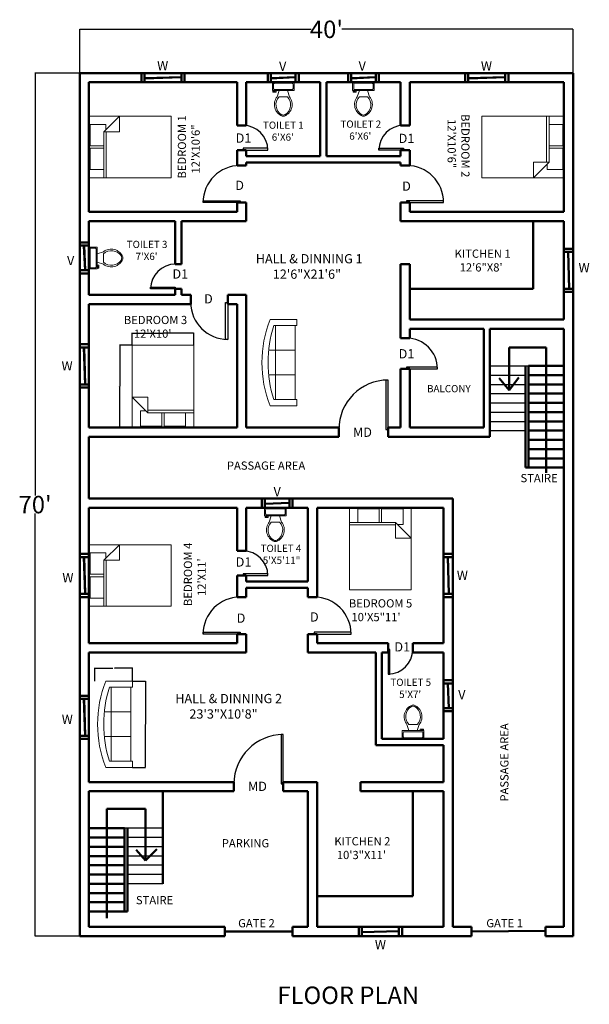
# Model space of a CAD drawing. Units: inches. Extents: x 9239 to 26065, y 6728 to 14611.
# Tile 5 of 12: x 11268 to 11822, y 6974 to 7933. Entities that reach past the tile are written whole.
import ezdxf

# ---------------------------------------------------------------- set-up
doc = ezdxf.new("R2010")
doc.units = ezdxf.units.IN
doc.header["$MEASUREMENT"] = 0
for name, color, linetype, lineweight in [('A-ANNO-DIMS', 2, 'Continuous', 18), ('A-ANNO-TEXT', 7, 'Continuous', 18), ('A-AREA-IDEN', 7, 'Continuous', 18), ('A-DOOR', 4, 'Continuous', 25), ('A-FLOR-FIXT', 8, 'Continuous', 18), ('A-FLOR-STRS', 3, 'Continuous', 25), ('A-FURN', 8, 'Continuous', 18), ('A-GLAZ', 4, 'Continuous', 25), ('A-WALL', 7, 'Continuous', 50)]:
    doc.layers.add(name, color=color, linetype=linetype, lineweight=lineweight)
doc.styles.get("Standard").update_dxf_attribs({"font": 'arial.ttf'})
doc.dimstyles.get("Standard").update_dxf_attribs({"dimtxt": 0.18, "dimasz": 0.18, "dimexe": 0.18, "dimexo": 0.0625, "dimgap": 0.09, "dimtad": 0, "dimtih": 1, "dimtoh": 1, "dimdec": 0, "dimzin": 0, "dimdsep": 46, "dimlunit": 3, "dimtxsty": 'Standard', "dimcen": 0.09, "dimadec": 0, "dimazin": 0, "dimtfac": 1, "dimtdec": 0, "dimtofl": 0, "dimtmove": 0, "dimatfit": 3, "dimfxl": 1, "dimtolj": 1, "dimtzin": 0, "dimarcsym": 0})

# ---------------------------------------------------------------- blocks, each defined once
blk = doc.blocks.new('Bed - Queen')
for p, q in [((0, -80.00003), (0, 0)), ((0, 0), (59.99999, 0)), ((59.99999, 0), (59.99999, -80.00003)), ((7.99999, -1.2), (28.79998, -1.2)), ((7.99999, -14.4), (7.99999, -1.2)), ((28.79998, -1.2), (28.79998, -14.4)), ((31.19999, -1.2), (51.99999, -1.2)), ((31.19999, -14.4), (31.19999, -1.2)), ((51.99999, -1.2), (51.99999, -16.4)), ((0, -14.4), (44.8, -14.4)), ((44.8, -16.8), (0, -16.8)), ((59.99999, -29.6), (44.8, -14.4)), ((44.8, -14.4), (44.8, -29.6)), ((51.99999, -16.4), (46.79936, -16.4)), ((44.8, -29.6), (59.99999, -29.6)), ((59.99999, -80.00003), (0, -80.00003))]:
    blk.add_line(p, q)
blk = doc.blocks.new('Sofa - Roundback 7 ft.')
for p, q in [((-12.00002, -32.4421), (-12.00003, -6.5971)), ((11.99997, -32.4421), (11.99998, -6.5971)), ((-36.000027, -34), (-36.000027, -11.4696)), ((-35.999844, -13.3819), (35.9998, -13.3819)), ((35.99998, -34), (35.99998, -11.4696)), ((-36.000027, -32.4421), (35.99998, -32.4421))]:
    blk.add_line(p, q)
for points in [[(-36.000027, -34), (-42.000027, -34), (-42.000027, -8)], [(41.99998, -8), (41.99998, -34), (35.99998, -34)]]:
    blk.add_lwpolyline(points)
for centre, radius, start, end in [((0, -114.25), 114.25, 68.43141, 111.5686), ((-0.00001, -127.1968), 121.1968, 72.72033, 107.2797)]:
    blk.add_arc(centre, radius, start, end)
blk = doc.blocks.new('Toilet - top')
for p, q in [((-10, -8.5), (-8, -8.5)), ((-10, -9.5), (-10, -8.5)), ((-7, -9.5), (-10, -9.5)), ((-8, -8.5), (-8, -8)), ((-7, -8), (-7, -9.5)), ((-4, -8), (-6, -14)), ((4, -8), (6, -14)), ((9.5, -6), (9.5, -2)), ((4, -14), (-4, -14))]:
    blk.add_line(p, q)
blk.add_lwpolyline([(10.5, -8), (10.5, 0), (-10.5, 0), (-10.5, -8)], close=True)
for points in [[(-9.5, -2), (-9.5, -6)], [(8.5, -1), (-8.5, -1)], [(-8.5, -7), (8.5, -7)]]:
    blk.add_lwpolyline(points)
for centre, radius, start, end in [((-8.62, -1.88), 0.884, 81.8699, 188.1301), ((-8.62, -6.12), 0.884, 171.8699, 278.1301), ((8.62, -1.88), 0.884, 351.8699, 98.1301), ((8.62, -6.12), 0.884, 261.8699, 8.1301), ((3.52, -21.58), 12.17, 141.46911, 247.97143), ((4.2, -21.82), 11.33, 136.36773, 238.94682), ((-3.52, -21.58), 12.17, 292.02843, 38.53071), ((-4.2, -21.82), 11.33, 301.05301, 43.63209), ((0, -27.88), 4, 245.73182, 294.26817), ((0, -29), 4, 254.86053, 285.13947)]:
    blk.add_arc(centre, radius, start, end)
blk = doc.blocks.new('*U16')
for p, q in [((0, 0), (0, -6)), ((-40, 0), (-40, -6))]:
    blk.add_line(p, q)
blk.add_lwpolyline([(0, 0), (0, 40), (-1.75, 40), (-1.75, 0)], close=True)
blk.add_arc((0, 0), 40, 90, 180)
blk = doc.blocks.new('*U11')
for p, q in [((0, 0), (0, -6)), ((-36, 0), (-36, -6))]:
    blk.add_line(p, q)
blk.add_lwpolyline([(0, 0), (0, 36), (-1.75, 36), (-1.75, 0)], close=True)
blk.add_arc((0, 0), 36, 90, 180)
blk = doc.blocks.new('*U25')
for p, q in [((-24, 0), (-24, -6)), ((0, 0), (0, -6))]:
    blk.add_line(p, q)
blk.add_lwpolyline([(0, 0), (0, 24), (-1.75, 24), (-1.75, 0)], close=True)
blk.add_arc((0, 0), 24, 90, 180)
blk = doc.blocks.new('*U24')
for p, q in [((0, 0), (0, 6)), ((24, 0), (24, 6))]:
    blk.add_line(p, q)
blk.add_lwpolyline([(0, 0), (0, -24), (1.75, -24), (1.75, 0)], close=True)
blk.add_arc((0, 0), 24, 270, 0)
blk = doc.blocks.new('*U14')
for p, q in [((-36, 0), (-36, 6)), ((0, 0), (0, 6))]:
    blk.add_line(p, q)
blk.add_lwpolyline([(0, 0), (0, -36), (-1.75, -36), (-1.75, 0)], close=True)
blk.add_arc((0, 0), 36, 180, 270)
blk = doc.blocks.new('*U29')
for p, q in [((-24, 0), (-24, 6)), ((0, 0), (0, 6))]:
    blk.add_line(p, q)
blk.add_lwpolyline([(0, 0), (0, -24), (-1.75, -24), (-1.75, 0)], close=True)
blk.add_arc((0, 0), 24, 180, 270)
blk = doc.blocks.new('*U26')
for p, q in [((-24, 0), (-24, -6)), ((0, 0), (0, -6))]:
    blk.add_line(p, q)
blk.add_lwpolyline([(0, 0), (0, 24), (-1.75, 24), (-1.75, 0)], close=True)
blk.add_arc((0, 0), 24, 90, 180)
blk = doc.blocks.new('*U30')
for p, q in [((0, 0), (0, -6)), ((-36, 0), (-36, -6))]:
    blk.add_line(p, q)
blk.add_lwpolyline([(0, 0), (0, 36), (-1.75, 36), (-1.75, 0)], close=True)
blk.add_arc((0, 0), 36, 90, 180)
blk = doc.blocks.new('*U28')
for p, q in [((0, 0), (0, -6)), ((-30, 0), (-30, -6))]:
    blk.add_line(p, q)
blk.add_lwpolyline([(0, 0), (0, 30), (-1.75, 30), (-1.75, 0)], close=True)
blk.add_arc((0, 0), 30, 90, 180)
blk = doc.blocks.new('*U27')
for p, q in [((-30, 0), (-30, 6)), ((0, 0), (0, 6))]:
    blk.add_line(p, q)
blk.add_lwpolyline([(0, 0), (0, -30), (-1.75, -30), (-1.75, 0)], close=True)
blk.add_arc((0, 0), 30, 180, 270)
blk = doc.blocks.new('*D31')
at = {"layer": 'A-ANNO-DIMS', "color": 0, "lineweight": -2, "transparency": 16777216}
for p, q in [((11326.22, 7880.73), (11326.22, 7923.38)), ((11326.4, 7923.2), (11551.37, 7923.2)), ((11806.04, 7923.2), (11581.08, 7923.2)), ((11806.22, 7880.73), (11806.22, 7923.38))]:
    blk.add_line(p, q, dxfattribs=at)
at = {"layer": 'A-ANNO-DIMS', "color": 0, "transparency": 16777216}
for points in [[(11326.4, 7923.23), (11326.4, 7923.17), (11326.22, 7923.2)], [(11806.04, 7923.23), (11806.04, 7923.17), (11806.22, 7923.2)]]:
    blk.add_solid(points, dxfattribs=at)
at = {"layer": 'Defpoints', "color": 0, "transparency": 16777216}
for p in [(11806.22, 7923.2), (11326.22, 7880.66), (11806.22, 7880.66)]:
    blk.add_point(p, dxfattribs=at)
at = {"layer": 'A-ANNO-DIMS', "color": 0, "transparency": 16777216, "insert": (11566.22, 7923.2), "char_height": 0.18, "attachment_point": 5}
blk.add_mtext("\\A1;{\\H94.44444x;40'}", dxfattribs=at)
blk = doc.blocks.new('*D32')
at = {"layer": 'A-ANNO-DIMS', "color": 0, "lineweight": -2, "transparency": 16777216}
for p, q in [((11326.16, 7880.66), (11282.62, 7880.66)), ((11282.8, 7880.48), (11282.8, 7469.43)), ((11282.8, 7040.84), (11282.8, 7451.89)), ((11326.16, 7040.66), (11282.62, 7040.66))]:
    blk.add_line(p, q, dxfattribs=at)
at = {"layer": 'A-ANNO-DIMS', "color": 0, "transparency": 16777216}
for points in [[(11282.77, 7880.48), (11282.83, 7880.48), (11282.8, 7880.66)], [(11282.77, 7040.84), (11282.83, 7040.84), (11282.8, 7040.66)]]:
    blk.add_solid(points, dxfattribs=at)
at = {"layer": 'Defpoints', "color": 0, "transparency": 16777216}
for p in [(11326.22, 7880.66), (11282.8, 7040.66), (11326.22, 7040.66)]:
    blk.add_point(p, dxfattribs=at)
at = {"layer": 'A-ANNO-DIMS', "color": 0, "transparency": 16777216, "insert": (11282.8, 7460.66), "char_height": 0.18, "width": 0.304, "attachment_point": 5}
blk.add_mtext("\\A1;{\\H94.44444x;70'}", dxfattribs=at)
blk = doc.blocks.new('WIN-36')
for p, q in [((0, 1), (36, 1)), ((0, 0.5), (36, 0.5)), ((0, 0), (36, 0))]:
    blk.add_line(p, q)
blk = doc.blocks.new('WIN-24')
for p, q in [((0, 1), (24, 1)), ((0, 0.5), (24, 0.5)), ((0, 0), (24, 0))]:
    blk.add_line(p, q)
blk = doc.blocks.new('*D46')
at = {"layer": 'A-ANNO-DIMS', "color": 0, "lineweight": -2, "transparency": 16777216}
for p, q in [((11377.16, 7615.66), (11365.04, 7615.66)), ((11365.22, 7615.48), (11365.22, 7575.85)), ((11365.22, 7535.84), (11365.22, 7575.48)), ((11377.16, 7535.66), (11365.04, 7535.66))]:
    blk.add_line(p, q, dxfattribs=at)
at = {"layer": 'A-ANNO-DIMS', "color": 0, "transparency": 16777216}
for points in [[(11365.19, 7615.48), (11365.25, 7615.48), (11365.22, 7615.66)], [(11365.19, 7535.84), (11365.25, 7535.84), (11365.22, 7535.66)]]:
    blk.add_solid(points, dxfattribs=at)
at = {"layer": 'Defpoints', "color": 0, "transparency": 16777216}
for p in [(11377.22, 7615.66), (11365.22, 7535.66), (11377.22, 7535.66)]:
    blk.add_point(p, dxfattribs=at)
at = {"layer": 'A-ANNO-DIMS', "color": 0, "transparency": 16777216, "insert": (11365.22, 7575.66), "char_height": 0.18, "attachment_point": 5}
blk.add_mtext('\\A1;QUEEN BED 6\'-8" TYP.', dxfattribs=at)
blk = doc.blocks.new('*D47')
at = {"layer": 'A-ANNO-DIMS', "color": 0, "lineweight": -2, "transparency": 16777216}
for p, q in [((11377.22, 7615.73), (11377.22, 7627.84)), ((11377.4, 7627.66), (11406.59, 7627.66)), ((11437.04, 7627.66), (11407.86, 7627.66)), ((11437.22, 7615.73), (11437.22, 7627.84))]:
    blk.add_line(p, q, dxfattribs=at)
at = {"layer": 'A-ANNO-DIMS', "color": 0, "transparency": 16777216}
for points in [[(11377.4, 7627.69), (11377.4, 7627.63), (11377.22, 7627.66)], [(11437.04, 7627.69), (11437.04, 7627.63), (11437.22, 7627.66)]]:
    blk.add_solid(points, dxfattribs=at)
at = {"layer": 'Defpoints', "color": 0, "transparency": 16777216}
for p in [(11377.22, 7627.66), (11377.22, 7615.66), (11437.22, 7615.66)]:
    blk.add_point(p, dxfattribs=at)
at = {"layer": 'A-ANNO-DIMS', "color": 0, "transparency": 16777216, "insert": (11407.22, 7627.66), "char_height": 0.18, "attachment_point": 5}
blk.add_mtext('\\A1;5\'-0" TYP.', dxfattribs=at)
blk = doc.blocks.new('*D54')
at = {"layer": 'A-ANNO-DIMS', "color": 0, "lineweight": -2, "transparency": 16777216}
for p, q in [((11377.64, 7288.88), (11390.36, 7288.88)), ((11390.18, 7288.7), (11390.18, 7247.06)), ((11390.18, 7205.06), (11390.18, 7246.7)), ((11377.64, 7204.88), (11390.36, 7204.88))]:
    blk.add_line(p, q, dxfattribs=at)
at = {"layer": 'A-ANNO-DIMS', "color": 0, "transparency": 16777216}
for points in [[(11390.15, 7288.7), (11390.21, 7288.7), (11390.18, 7288.88)], [(11390.15, 7205.06), (11390.21, 7205.06), (11390.18, 7204.88)]]:
    blk.add_solid(points, dxfattribs=at)
at = {"layer": 'Defpoints', "color": 0, "transparency": 16777216}
for p in [(11377.58, 7288.88), (11390.18, 7288.88), (11377.58, 7204.88)]:
    blk.add_point(p, dxfattribs=at)
at = {"layer": 'A-ANNO-DIMS', "color": 0, "transparency": 16777216, "insert": (11390.18, 7246.88), "char_height": 0.18, "attachment_point": 5}
blk.add_mtext('\\A1;SOFA 7\'-0" TYP.', dxfattribs=at)
blk = doc.blocks.new('*D55')
at = {"layer": 'A-ANNO-DIMS', "color": 0, "lineweight": -2, "transparency": 16777216}
for p, q in [((11340.91, 7288.94), (11340.91, 7301.66)), ((11341.09, 7301.48), (11358.4, 7301.48)), ((11377.4, 7301.48), (11360.09, 7301.48)), ((11377.58, 7288.94), (11377.58, 7301.66))]:
    blk.add_line(p, q, dxfattribs=at)
at = {"layer": 'A-ANNO-DIMS', "color": 0, "transparency": 16777216}
for points in [[(11341.09, 7301.51), (11341.09, 7301.45), (11340.91, 7301.48)], [(11377.4, 7301.51), (11377.4, 7301.45), (11377.58, 7301.48)]]:
    blk.add_solid(points, dxfattribs=at)
at = {"layer": 'Defpoints', "color": 0, "transparency": 16777216}
for p in [(11340.91, 7301.48), (11340.91, 7288.88), (11377.58, 7288.88)]:
    blk.add_point(p, dxfattribs=at)
at = {"layer": 'A-ANNO-DIMS', "color": 0, "transparency": 16777216, "insert": (11359.25, 7301.48), "char_height": 0.18, "attachment_point": 5}
blk.add_mtext('\\A1;3\'-0 1/2" TYP.', dxfattribs=at)

msp = doc.modelspace()

# ---------------------------------------------------------------- linework, layer by layer
at = {"layer": 'A-FLOR-STRS'}
for p, q in [((11725.22, 7595.66), (11762.72, 7595.66)), ((11725.22, 7586.66), (11759.72, 7586.66)), ((11725.22, 7577.66), (11759.72, 7577.66)), ((11725.22, 7568.66), (11759.72, 7568.66)), ((11725.22, 7559.66), (11759.72, 7559.66)), ((11725.22, 7550.66), (11759.72, 7550.66)), ((11725.22, 7541.66), (11759.72, 7541.66)), ((11725.22, 7532.66), (11759.72, 7532.66)), ((11407.22, 7145.66), (11369.72, 7145.66)), ((11407.22, 7136.66), (11372.72, 7136.66)), ((11407.22, 7127.66), (11372.72, 7127.66)), ((11407.22, 7118.66), (11372.72, 7118.66)), ((11407.22, 7109.66), (11372.72, 7109.66)), ((11407.22, 7100.66), (11372.72, 7100.66)), ((11407.22, 7091.66), (11372.72, 7091.66))]:
    msp.add_line(p, q, dxfattribs=at)
at = {"layer": 'A-WALL'}
for p, q in [((11326.22, 7880.66), (11806.22, 7880.66)), ((11326.22, 7040.66), (11326.22, 7880.66)), ((11386.22, 7871.66), (11386.22, 7880.66)), ((11389.22, 7871.66), (11389.22, 7880.66)), ((11425.22, 7871.66), (11425.22, 7880.66)), ((11428.22, 7871.66), (11428.22, 7880.66)), ((11509.22, 7871.66), (11509.22, 7880.66)), ((11512.22, 7871.66), (11512.22, 7880.66)), ((11536.22, 7871.66), (11536.22, 7880.66)), ((11539.22, 7871.66), (11539.22, 7880.66)), ((11587.22, 7871.66), (11587.22, 7880.66)), ((11590.22, 7871.66), (11590.22, 7880.66)), ((11614.22, 7871.66), (11614.22, 7880.66)), ((11617.22, 7871.66), (11617.22, 7880.66)), ((11701.22, 7871.66), (11701.22, 7880.66)), ((11704.22, 7871.66), (11704.22, 7880.66)), ((11740.22, 7871.66), (11740.22, 7880.66)), ((11743.22, 7871.66), (11743.22, 7880.66)), ((11806.22, 7880.66), (11806.22, 7040.66)), ((11335.22, 7871.66), (11479.22, 7871.66)), ((11335.22, 7745.66), (11335.22, 7871.66)), ((11479.22, 7829.66), (11479.22, 7871.66)), ((11488.22, 7829.66), (11488.22, 7871.66)), ((11488.22, 7871.66), (11560.22, 7871.66)), ((11560.22, 7799.66), (11560.22, 7871.66)), ((11566.22, 7799.66), (11566.22, 7871.66)), ((11566.22, 7871.66), (11638.22, 7871.66)), ((11638.22, 7829.66), (11638.22, 7871.66)), ((11647.22, 7829.66), (11647.22, 7871.66)), ((11647.22, 7871.66), (11797.22, 7871.66)), ((11797.22, 7871.66), (11797.22, 7745.66)), ((11479.22, 7829.66), (11488.22, 7829.66)), ((11638.22, 7829.66), (11647.22, 7829.66)), ((11479.22, 7790.66), (11479.22, 7805.66)), ((11479.22, 7805.66), (11488.22, 7805.66)), ((11488.22, 7799.66), (11488.22, 7805.66)), ((11638.22, 7805.66), (11647.22, 7805.66)), ((11638.22, 7799.66), (11638.22, 7805.66)), ((11647.22, 7790.66), (11647.22, 7805.66)), ((11479.22, 7790.66), (11488.22, 7790.66)), ((11488.22, 7799.66), (11560.22, 7799.66)), ((11488.22, 7793.66), (11638.22, 7793.66)), ((11488.22, 7790.66), (11488.22, 7793.66)), ((11566.22, 7799.66), (11638.22, 7799.66)), ((11638.22, 7790.66), (11638.22, 7793.66)), ((11638.22, 7790.66), (11647.22, 7790.66)), ((11479.22, 7745.66), (11479.22, 7754.66)), ((11479.22, 7754.66), (11488.22, 7754.66)), ((11488.22, 7736.66), (11488.22, 7754.66)), ((11638.22, 7736.66), (11638.22, 7754.66)), ((11638.22, 7754.66), (11647.22, 7754.66)), ((11647.22, 7745.66), (11647.22, 7754.66)), ((11335.22, 7745.66), (11479.22, 7745.66)), ((11647.22, 7745.66), (11797.22, 7745.66)), ((11335.22, 7736.66), (11419.22, 7736.66)), ((11335.22, 7664.66), (11335.22, 7736.66)), ((11419.22, 7694.66), (11419.22, 7736.66)), ((11425.22, 7694.66), (11425.22, 7736.66)), ((11425.22, 7736.66), (11488.22, 7736.66)), ((11638.22, 7736.66), (11797.22, 7736.66)), ((11767.22, 7736.66), (11767.22, 7670.66)), ((11797.22, 7736.66), (11797.22, 7640.66)), ((11335.22, 7715.66), (11326.22, 7715.66)), ((11335.22, 7712.66), (11326.22, 7712.66)), ((11797.22, 7709.66), (11806.22, 7709.66)), ((11797.22, 7706.66), (11806.22, 7706.66)), ((11335.22, 7688.66), (11326.22, 7688.66)), ((11335.22, 7685.66), (11326.22, 7685.66)), ((11419.22, 7694.66), (11425.22, 7694.66)), ((11638.22, 7694.66), (11647.22, 7694.66)), ((11638.22, 7622.66), (11638.22, 7694.66)), ((11647.22, 7640.66), (11647.22, 7694.66)), ((11419.22, 7664.66), (11419.22, 7670.66)), ((11419.22, 7670.66), (11425.22, 7670.66)), ((11425.22, 7664.66), (11425.22, 7670.66)), ((11647.22, 7670.66), (11767.22, 7670.66)), ((11797.22, 7670.66), (11806.22, 7670.66)), ((11797.22, 7667.66), (11806.22, 7667.66)), ((11335.22, 7664.66), (11419.22, 7664.66)), ((11425.22, 7664.66), (11434.22, 7664.66)), ((11434.22, 7655.66), (11434.22, 7664.66)), ((11470.22, 7655.66), (11470.22, 7664.66)), ((11470.22, 7664.66), (11488.22, 7664.66)), ((11488.22, 7535.66), (11488.22, 7664.66)), ((11335.22, 7655.66), (11434.22, 7655.66)), ((11335.22, 7535.66), (11335.22, 7655.66)), ((11470.22, 7655.66), (11479.22, 7655.66)), ((11479.22, 7535.66), (11479.22, 7655.66)), ((11647.22, 7640.66), (11797.22, 7640.66)), ((11647.22, 7631.66), (11719.22, 7631.66)), ((11647.22, 7622.66), (11647.22, 7631.66)), ((11719.22, 7631.66), (11719.22, 7535.66)), ((11725.22, 7631.66), (11725.22, 7526.66)), ((11725.22, 7631.66), (11797.22, 7631.66)), ((11797.22, 7631.66), (11797.22, 7049.66)), ((11638.22, 7622.66), (11647.22, 7622.66)), ((11335.22, 7616.66), (11326.22, 7616.66)), ((11335.22, 7613.66), (11326.22, 7613.66)), ((11779.97, 7613.53), (11743.89, 7613.53)), ((11743.89, 7613.53), (11743.89, 7571.97)), ((11779.97, 7491.45), (11779.97, 7613.53)), ((11638.22, 7571.66), (11638.22, 7592.66)), ((11638.22, 7592.66), (11647.22, 7592.66)), ((11647.22, 7571.66), (11647.22, 7592.66)), ((11759.72, 7595.66), (11759.72, 7496.66)), ((11762.72, 7595.66), (11762.72, 7496.66)), ((11762.72, 7595.66), (11797.22, 7595.66)), ((11743.89, 7571.97), (11734.18, 7583.85)), ((11743.89, 7571.97), (11753.43, 7584.48)), ((11762.72, 7586.66), (11797.22, 7586.66)), ((11335.22, 7577.66), (11326.22, 7577.66)), ((11335.22, 7574.66), (11326.22, 7574.66)), ((11638.22, 7535.66), (11638.22, 7571.66)), ((11647.22, 7535.66), (11647.22, 7571.66)), ((11762.72, 7577.66), (11797.22, 7577.66)), ((11762.72, 7568.66), (11797.22, 7568.66)), ((11762.72, 7559.66), (11797.22, 7559.66)), ((11762.72, 7550.66), (11797.22, 7550.66)), ((11762.72, 7541.66), (11797.22, 7541.66)), ((11335.22, 7535.66), (11479.22, 7535.66)), ((11488.22, 7535.66), (11578.22, 7535.66)), ((11578.22, 7526.66), (11578.22, 7535.66)), ((11626.22, 7526.66), (11626.22, 7535.66)), ((11626.22, 7535.66), (11638.22, 7535.66)), ((11647.22, 7535.66), (11719.22, 7535.66)), ((11762.72, 7532.66), (11797.22, 7532.66)), ((11335.22, 7526.66), (11578.22, 7526.66)), ((11335.22, 7466.66), (11335.22, 7526.66)), ((11626.22, 7526.66), (11725.22, 7526.66)), ((11762.72, 7523.66), (11797.22, 7523.66)), ((11762.72, 7514.66), (11797.22, 7514.66)), ((11762.72, 7505.66), (11797.22, 7505.66)), ((11759.72, 7496.66), (11797.22, 7496.66)), ((11335.22, 7466.66), (11689.22, 7466.66)), ((11503.22, 7457.66), (11503.22, 7466.66)), ((11506.22, 7457.66), (11506.22, 7466.66)), ((11530.22, 7457.66), (11530.22, 7466.66)), ((11533.22, 7457.66), (11533.22, 7466.66)), ((11689.22, 7466.66), (11689.22, 7049.66)), ((11335.22, 7457.66), (11479.22, 7457.66)), ((11335.22, 7325.66), (11335.22, 7457.66)), ((11476.22, 7457.66), (11479.22, 7457.66)), ((11479.22, 7415.66), (11479.22, 7457.66)), ((11488.22, 7415.66), (11488.22, 7457.66)), ((11488.22, 7457.66), (11548.22, 7457.66)), ((11548.22, 7385.66), (11548.22, 7457.66)), ((11557.22, 7370.66), (11557.22, 7457.66)), ((11557.22, 7457.66), (11680.22, 7457.66)), ((11680.22, 7457.66), (11680.22, 7325.66)), ((11335.22, 7412.66), (11326.22, 7412.66)), ((11335.22, 7409.66), (11326.22, 7409.66)), ((11479.22, 7415.66), (11488.22, 7415.66)), ((11680.22, 7412.66), (11689.22, 7412.66)), ((11680.22, 7409.66), (11689.22, 7409.66)), ((11479.22, 7370.66), (11479.22, 7391.66)), ((11479.22, 7391.66), (11488.22, 7391.66)), ((11488.22, 7385.66), (11488.22, 7391.66)), ((11488.22, 7385.66), (11548.22, 7385.66)), ((11488.22, 7379.66), (11548.22, 7379.66)), ((11488.22, 7370.66), (11488.22, 7379.66)), ((11548.22, 7370.66), (11548.22, 7379.66)), ((11335.22, 7373.66), (11326.22, 7373.66)), ((11335.22, 7370.66), (11326.22, 7370.66)), ((11479.22, 7370.66), (11488.22, 7370.66)), ((11548.22, 7370.66), (11557.22, 7370.66)), ((11680.22, 7373.66), (11689.22, 7373.66)), ((11680.22, 7370.66), (11689.22, 7370.66)), ((11479.22, 7334.66), (11488.22, 7334.66)), ((11479.22, 7325.66), (11479.22, 7334.66)), ((11488.22, 7316.66), (11488.22, 7334.66)), ((11548.22, 7316.66), (11548.22, 7334.66)), ((11548.22, 7334.66), (11557.22, 7334.66)), ((11557.22, 7325.66), (11557.22, 7334.66)), ((11335.22, 7325.66), (11479.22, 7325.66)), ((11557.22, 7325.66), (11626.22, 7325.66)), ((11626.22, 7325.66), (11626.22, 7316.66)), ((11650.22, 7325.66), (11650.22, 7316.66)), ((11650.22, 7325.66), (11680.22, 7325.66)), ((11335.22, 7316.66), (11488.22, 7316.66)), ((11335.22, 7190.66), (11335.22, 7316.66)), ((11548.22, 7316.66), (11614.22, 7316.66)), ((11614.22, 7316.66), (11614.22, 7226.66)), ((11620.22, 7316.66), (11620.22, 7232.66)), ((11620.22, 7316.66), (11626.22, 7316.66)), ((11650.22, 7316.66), (11680.22, 7316.66)), ((11680.22, 7316.66), (11680.22, 7232.66)), ((11680.22, 7289.66), (11689.22, 7289.66)), ((11680.22, 7286.66), (11689.22, 7286.66)), ((11335.22, 7274.66), (11326.22, 7274.66)), ((11335.22, 7271.66), (11326.22, 7271.66)), ((11680.22, 7262.66), (11689.22, 7262.66)), ((11680.22, 7259.66), (11689.22, 7259.66)), ((11335.22, 7235.66), (11326.22, 7235.66)), ((11335.22, 7232.66), (11326.22, 7232.66)), ((11614.22, 7226.66), (11680.22, 7226.66)), ((11620.22, 7232.66), (11680.22, 7232.66)), ((11680.22, 7226.66), (11680.22, 7190.66)), ((11476.22, 7190.66), (11335.22, 7190.66)), ((11476.22, 7181.66), (11476.22, 7190.66)), ((11557.22, 7190.66), (11524.22, 7190.66)), ((11557.22, 7190.66), (11524.22, 7190.66)), ((11524.22, 7181.66), (11524.22, 7190.66)), ((11557.22, 7049.66), (11557.22, 7190.66)), ((11680.22, 7190.66), (11599.22, 7190.66)), ((11599.22, 7181.66), (11599.22, 7190.66)), ((11335.22, 7049.66), (11335.22, 7181.66)), ((11476.22, 7181.66), (11335.22, 7181.66)), ((11407.22, 7091.66), (11407.22, 7181.66)), ((11548.22, 7181.66), (11524.22, 7181.66)), ((11548.22, 7049.66), (11548.22, 7181.66)), ((11680.22, 7181.66), (11599.22, 7181.66)), ((11650.22, 7181.66), (11650.22, 7079.66)), ((11680.22, 7181.66), (11680.22, 7049.66)), ((11352.47, 7058.27), (11352.47, 7164.58)), ((11352.47, 7164.58), (11390.09, 7164.58)), ((11390.09, 7164.58), (11390.09, 7114.39)), ((11369.72, 7145.66), (11335.22, 7145.66)), ((11369.72, 7064.66), (11369.72, 7145.66)), ((11372.72, 7064.66), (11372.72, 7145.66)), ((11369.72, 7136.66), (11335.22, 7136.66)), ((11369.72, 7127.66), (11335.22, 7127.66)), ((11390.09, 7114.39), (11381, 7124.81)), ((11390.09, 7114.39), (11401.25, 7125.18)), ((11369.72, 7118.66), (11335.22, 7118.66)), ((11369.72, 7109.66), (11335.22, 7109.66)), ((11369.72, 7100.66), (11335.22, 7100.66)), ((11369.72, 7091.66), (11335.22, 7091.66)), ((11369.72, 7082.66), (11335.22, 7082.66)), ((11369.72, 7073.66), (11335.22, 7073.66)), ((11650.22, 7079.66), (11557.22, 7079.66)), ((11372.72, 7064.66), (11335.22, 7064.66)), ((11467.22, 7049.66), (11335.22, 7049.66)), ((11467.22, 7049.66), (11467.22, 7040.66)), ((11467.22, 7045.16), (11533.22, 7045.16)), ((11548.22, 7049.66), (11533.22, 7049.66)), ((11533.22, 7040.66), (11533.22, 7049.66)), ((11680.22, 7049.66), (11557.22, 7049.66)), ((11597.72, 7049.66), (11597.72, 7040.66)), ((11600.72, 7049.66), (11600.72, 7040.66)), ((11636.72, 7049.66), (11636.72, 7040.66)), ((11639.72, 7049.66), (11639.72, 7040.66)), ((11707.22, 7049.66), (11689.22, 7049.66)), ((11707.22, 7049.66), (11707.22, 7040.66)), ((11707.22, 7045.16), (11779.22, 7046)), ((11797.22, 7049.66), (11779.22, 7049.66)), ((11779.22, 7049.66), (11779.22, 7040.66)), ((11467.22, 7040.66), (11326.22, 7040.66)), ((11707.22, 7040.66), (11533.22, 7040.66)), ((11806.22, 7040.66), (11779.22, 7040.66))]:
    msp.add_line(p, q, dxfattribs=at)

# ---------------------------------------------------------------- block references
at = {"layer": 'A-DOOR', "rotation": 270}
for name, p in [('*U26', (11485.22, 7805.66)), ('*U29', (11641.22, 7805.66)), ('*U14', (11482.22, 7754.66)), ('*U30', (11644.22, 7754.66)), ('*U29', (11419.22, 7670.66)), ('*U28', (11644.22, 7592.66)), ('*U25', (11485.22, 7391.66)), ('*U14', (11482.22, 7334.66)), ('*U11', (11554.22, 7334.66))]:
    msp.add_blockref(name, p, dxfattribs=at)
at = {"layer": 'A-DOOR', "xscale": 1.199999999999999, "yscale": 1.199999999999999, "zscale": 1.199999999999999}
for name, p in [('*U27', (11470.22, 7657.46)), ('*U16', (11626.22, 7533.86)), ('*U16', (11524.22, 7188.86))]:
    msp.add_blockref(name, p, dxfattribs=at)
at = {"layer": 'A-DOOR'}
msp.add_blockref('*U24', (11626.22, 7319.66), dxfattribs=at)
at = {"layer": 'A-FLOR-FIXT'}
for p in [(11524.22, 7871.66), (11602.22, 7871.66), (11516.56, 7457.66)]:
    msp.add_blockref('Toilet - top', p, dxfattribs=at)
for p, rotation in [((11335.22, 7700.66), 89.99999999999999), ((11650.49, 7232.66), 180)]:
    msp.add_blockref('Toilet - top', p, dxfattribs=dict(at, rotation=rotation))
at = {"layer": 'A-FURN'}
for name, p, rotation in [('Bed - Queen', (11335.22, 7778.66), 90), ('Bed - Queen', (11797.22, 7838.66), 270), ('Sofa - Roundback 7 ft.', (11503.43, 7598.82), 90), ('Bed - Queen', (11437.22, 7535.66), 180), ('Bed - Queen', (11335.22, 7361.66), 90), ('Sofa - Roundback 7 ft.', (11343.58, 7246.88), 90)]:
    msp.add_blockref(name, p, dxfattribs=dict(at, rotation=rotation))
msp.add_blockref('Bed - Queen', (11588.72, 7457.66), dxfattribs=at)
at = {"layer": 'A-GLAZ'}
for name, p, rotation in [('WIN-36', (11389.24, 7875.16), 1.591140271200308), ('WIN-24', (11512.26, 7875.16), 2.385944030397281), ('WIN-24', (11590.26, 7875.16), 2.385944030397281), ('WIN-36', (11704.24, 7875.16), 1.591140271200308), ('WIN-24', (11329.72, 7712.63), 272.3859440303975), ('WIN-36', (11800.72, 7706.64), 271.5911402712003), ('WIN-36', (11329.72, 7613.64), 271.5911402711714), ('WIN-24', (11506.26, 7461.16), 2.385944030397281), ('WIN-36', (11329.72, 7409.64), 271.5911402712003), ('WIN-36', (11683.72, 7409.64), 271.5911402712003), ('WIN-24', (11683.72, 7286.63), 272.3859440303888), ('WIN-36', (11329.72, 7271.64), 271.5911402712003), ('WIN-36', (11600.74, 7044.16), 1.591140271200308)]:
    msp.add_blockref(name, p, dxfattribs=dict(at, rotation=rotation))

# ---------------------------------------------------------------- texts
at = {"layer": 'A-ANNO-TEXT', "attachment_point": 1}
for s, width, insert, char_height in [('W', 497.8283, (11401.53, 7892.38), 9), ('V', 497.8283, (11520.11, 7891.73), 9), ('V', 497.8283, (11597.49, 7892.09), 9), ('W', 497.8283, (11716.47, 7892.07), 9), ('D1', 497.8283, (11477.91, 7821.86), 9), ('D1', 497.8283, (11636.44, 7821.54), 9), ('D', 497.8283, (11477.53, 7775.87), 9), ('D', 497.8283, (11639.85, 7775.07), 9), ('V', 497.8283, (11313.87, 7702.73), 9), ('W', 497.8283, (11811.45, 7695.71), 9), ('D1', 497.8283, (11416.43, 7689.62), 9), ('D', 497.8283, (11447.18, 7665.41), 9), ('D1', 497.8283, (11636.44, 7611.93), 9), ('W', 497.8283, (11308.54, 7600.18), 9), ('MD', 497.8283, (11592.03, 7535.6), 9), ('V', 497.8283, (11514.76, 7477.82), 9), ('D1', 497.8283, (11477.97, 7409.29), 9), ('W', 497.8283, (11309.35, 7394.01), 9), ('W', 497.8283, (11693.04, 7396.34), 9), ('D', 497.8283, (11478.91, 7354.66), 9), ('D', 497.8283, (11550.2, 7355.84), 9), ('D1', 497.8283, (11632.3, 7326.7), 9), ('V', 497.8283, (11694.37, 7280.09), 9), ('W', 497.8283, (11308.73, 7256.28), 9), ('MD', 497.8283, (11489.88, 7190.97), 9), ('W', 497.8283, (11613.35, 7036.88), 9), ('FLOOR PLAN', 2149.001, (11518.52, 6991.64), 17)]:
    msp.add_mtext_dynamic_manual_height_columns(s, width=width, gutter_width=1, heights=[0], dxfattribs=dict(at, insert=insert, char_height=char_height))
at = {"layer": 'A-AREA-IDEN', "char_height": 8, "attachment_point": 1}
for s, width, heights, insert, rotation in [('BEDROOM 1\\P  12\'X10\'6"', 517.3321, [0], (11421.65, 7777.97), 90), ('BEDROOM 2 \\P  12\'X10\'6"', 567.5122, [0], (11705.38, 7840.74), 270), ("BEDROOM 4\\P    12'X11'", 1710.3911, [0], (11427.49, 7361.97), 90), ('PASSAGE AREA', 151.4238, [8.27], (11735.3, 7171.65), 90)]:
    msp.add_mtext_dynamic_manual_height_columns(s, width=width, gutter_width=1, heights=heights, dxfattribs=dict(at, insert=insert, rotation=rotation))
at = {"layer": 'A-AREA-IDEN', "attachment_point": 1}
for s, width, insert, char_height in [("TOILET 1\\P    6'X6'", 410.2419, (11504.49, 7833.42), 7), ("TOILET 2\\P    6'X6'", 410.2419, (11579.85, 7834.45), 7), ("TOILET 3\\P    7'X6'", 380.4249, (11371.94, 7717.39), 7), ('HALL & DINNING 1\\P      12\'6"X21\'6"', 2531.1126, (11497.53, 7704.43), 9), ('KITCHEN 1\\P  12\'6"X8\'', 631.7999, (11690.93, 7708.86), 8), ("BEDROOM 3\\P    12'X10'", 1285.9943, (11369.16, 7644.34), 8), ('BALCONY', 384.0781, (11664.08, 7576.98), 7), ('PASSAGE AREA', 151.4238, (11469.39, 7502.6), 8), ('STAIRE', 151.4238, (11754.96, 7490.46), 8), ('TOILET 4\\P 5\'X5\'11"', 1805.8319, (11502.17, 7421.6), 7), ('BEDROOM 5\\P 10\'X5"11\'', 2010.6578, (11588.08, 7368.54), 8), ("TOILET 5\\P    5'X7'", 1821.3046, (11628.41, 7291.19), 7), ('HALL & DINNING 2\\P     23\'3"X10\'8"', 1069.5419, (11419.16, 7276.4), 9), ('PARKING', 151.4238, (11464.41, 7135.06), 8), ('KITCHEN 2\\P 10\'3"X11\'', 651.3748, (11573.91, 7137), 8), ('STAIRE', 151.4238, (11380.89, 7079.7), 8), ('GATE 2', 151.4238, (11480.34, 7057.23), 8), ('GATE 1', 151.4238, (11721.71, 7057.28), 8)]:
    msp.add_mtext_dynamic_manual_height_columns(s, width=width, gutter_width=1, heights=[0], dxfattribs=dict(at, insert=insert, char_height=char_height))

# ---------------------------------------------------------------- dimensions: what is measured, and where the dimension line sits
at = {"layer": 'A-ANNO-DIMS'}
dim = msp.add_linear_dim(base=(11806.22, 7923.2), p1=(11326.22, 7880.66), p2=(11806.22, 7880.66), text='{\\H94.44444x;<>}', dimstyle='Standard', override={"dimclrd": 0, "dimclre": 0, "dimclrt": 0}, dxfattribs=at)
dim.commit()
dim.dimension.update_dxf_attribs({"geometry": '*D31', "text_midpoint": (11566.22, 7923.2)})
for base, p1, p2, angle, text, override, picture, middle in [((11282.8, 7040.66), (11326.22, 7880.66), (11326.22, 7040.66), 90, '{\\H94.44444x;<>}', {"dimclrd": 0, "dimclre": 0, "dimclrt": 0}, '*D32', (11282.8, 7460.66)), ((11377.22, 7627.66), (11437.22, 7615.66), (11377.22, 7615.66), 180, '<> TYP.', {"dimdec": 1, "dimlfac": 1, "dimrnd": 0, "dimzin": 1, "dimdsep": 46, "dimlunit": 4, "dimfrac": 2}, '*D47', (11407.22, 7627.66)), ((11365.22, 7535.66), (11377.22, 7615.66), (11377.22, 7535.66), 270, 'QUEEN BED <> TYP.', {"dimdec": 1, "dimlfac": 1, "dimrnd": 0, "dimzin": 1, "dimdsep": 46, "dimlunit": 4, "dimfrac": 2}, '*D46', (11365.22, 7575.66)), ((11340.91, 7301.48), (11377.58, 7288.88), (11340.91, 7288.88), 180, '<> TYP.', {"dimdec": 1, "dimlfac": 1, "dimrnd": 0, "dimzin": 1, "dimdsep": 46, "dimlunit": 4, "dimfrac": 2}, '*D55', (11359.25, 7301.48)), ((11390.18, 7288.88), (11377.58, 7204.88), (11377.58, 7288.88), 90, 'SOFA <> TYP.', {"dimdec": 1, "dimlfac": 1, "dimrnd": 0, "dimzin": 1, "dimdsep": 46, "dimlunit": 4, "dimfrac": 2}, '*D54', (11390.18, 7246.88))]:
    dim = msp.add_linear_dim(base=base, p1=p1, p2=p2, angle=angle, text=text, dimstyle='Standard', override=override, dxfattribs=at)
    dim.commit()
    dim.dimension.update_dxf_attribs({"geometry": picture, "text_midpoint": middle})

doc.saveas('drawing.dxf')
